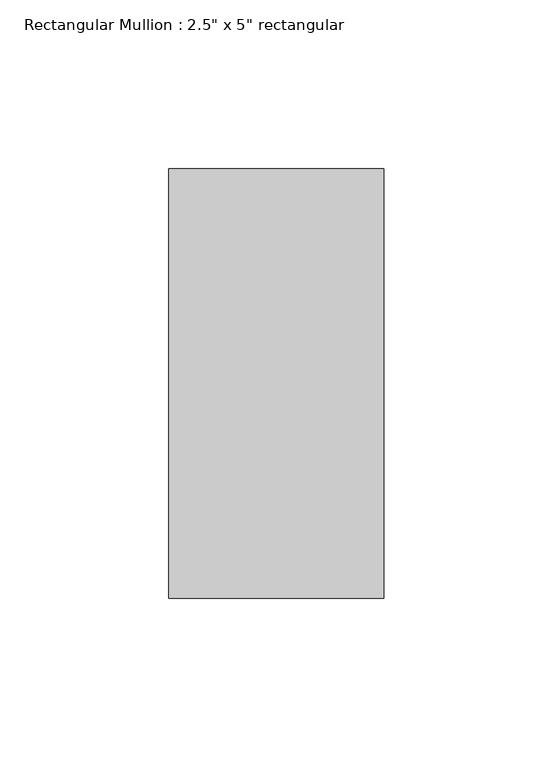
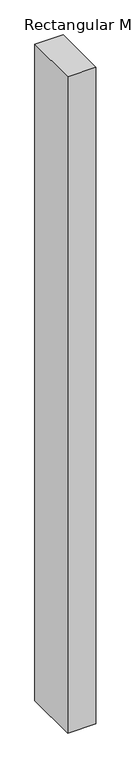
"""IFC4 building model written with IfcOpenShell, lengths in millimetres: member geometry."""

from ifc_helpers import new_model, si_unit, frame, origin, place, context, project, spatial, polyline, outline, extrude, source, transform, mapped, element, save


def member_4eea421a(model_context):
    return source(origin(), model_context, "Body", "SweptSolid", [
        extrude(outline(polyline([(0.0, 63.5), (0.0, -63.5), (-63.5, -63.5), (-63.5, 63.5), (0.0, 63.5)])), frame((0.0, 0.0, -1557.3709712), z_axis=(0.0, 0.0, 1.0), x_axis=(1.0, 0.0, 0.0)), (0.0, 0.0, 1.0), 1557.3709712),
    ])


if __name__ == "__main__":
    model = new_model("IFC4")
    model_context = context("Model", 3, world=origin())
    ifc_project = project(units=[si_unit("LENGTHUNIT", "METRE", prefix="MILLI")], contexts=[model_context])
    site = spatial("IfcSite", under=ifc_project)
    building = spatial("IfcBuilding", under=site)
    placement = place(None, origin())
    member_shape = member_4eea421a(model_context)
    element("IfcMember", 1, ObjectType="Rectangular Mullion : 2.5\" x 5\" rectangular", at=placement, inside=building, context=model_context, shape_type="MappedRepresentation", body=[
        mapped(member_shape, transform((0.0, 0.0, 0.0), x_axis=(1.0, 0.0, 0.0), y_axis=(0.0, 1.0, 0.0), z_axis=(0.0, 0.0, 1.0))),
    ])
    save(model, "model.ifc")

# Revit data of these elements
# Type "Rectangular Mullion : 2.5\" x 5\" rectangular"
#   built-in parameter 1007304 = 0.416667 (stored number, unit not read)
#   built-in parameter 1007301 = 0.104167 (stored number, unit not read)
#   built-in parameter 1007300 = 0.104167 (stored number, unit not read)
# Element 1 (IfcMember, "Rectangular Mullion : 2.5\" x 5\" rectangular")
#   Materials on its faces: "Aluminum"
# Materials
#   "Aluminum": class "Metal", colour RGB 247 247 247, transparency 0, Description = "Aluminum 6061", Cost = 0
